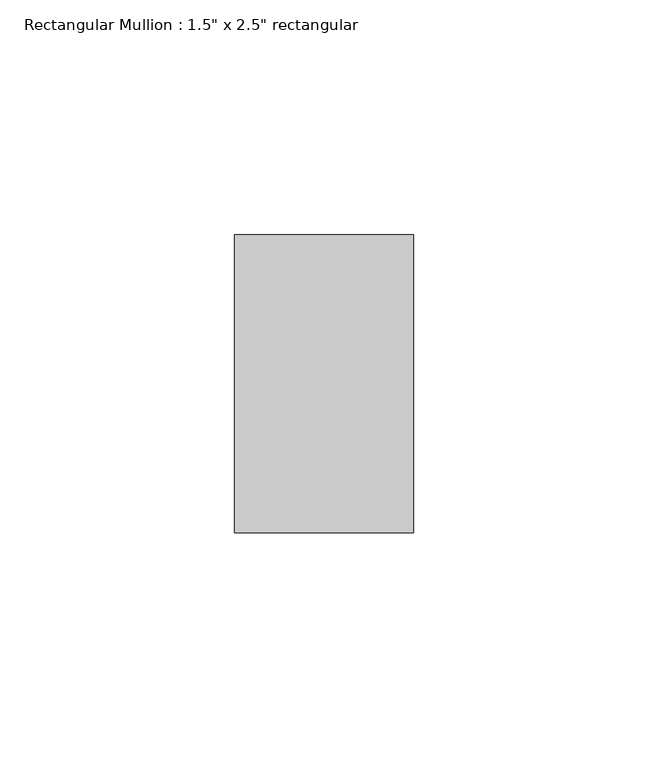
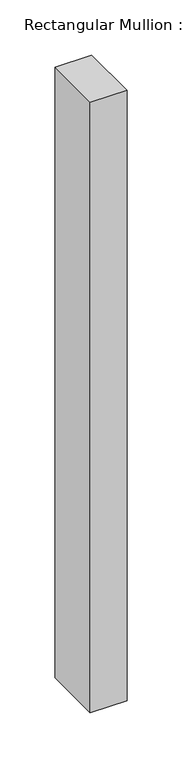
"""IFC4 building model written with IfcOpenShell, lengths in millimetres: member geometry."""

from ifc_helpers import new_model, si_unit, frame, origin, place, context, project, spatial, polyline, outline, extrude, source, transform, mapped, element, save


def member_7f78ed44(model_context):
    return source(origin(), model_context, "Body", "SweptSolid", [
        extrude(outline(polyline([(0.0, 31.75), (0.0, -31.75), (-38.1, -31.75), (-38.1, 31.75), (0.0, 31.75)])), frame((0.0, 0.0, -673.1), z_axis=(0.0, 0.0, 1.0), x_axis=(1.0, 0.0, 0.0)), (0.0, 0.0, 1.0), 673.1),
    ])


if __name__ == "__main__":
    model = new_model("IFC4")
    model_context = context("Model", 3, world=origin())
    ifc_project = project(units=[si_unit("LENGTHUNIT", "METRE", prefix="MILLI")], contexts=[model_context])
    site = spatial("IfcSite", under=ifc_project)
    building = spatial("IfcBuilding", under=site)
    placement = place(None, origin())
    member_shape = member_7f78ed44(model_context)
    element("IfcMember", 1, ObjectType="Rectangular Mullion : 1.5\" x 2.5\" rectangular", at=placement, inside=building, context=model_context, shape_type="MappedRepresentation", body=[
        mapped(member_shape, transform((0.0, 0.0, 0.0), x_axis=(1.0, 0.0, 0.0), y_axis=(0.0, 1.0, 0.0), z_axis=(0.0, 0.0, 1.0))),
    ])
    save(model, "model.ifc")

# Revit data of these elements
# Type "Rectangular Mullion : 1.5\" x 2.5\" rectangular"
#   built-in parameter 1007304 = 0.208333 (stored number, unit not read)
#   built-in parameter 1007301 = 0.0625 (stored number, unit not read)
#   built-in parameter 1007300 = 0.0625 (stored number, unit not read)
# Element 1 (IfcMember, "Rectangular Mullion : 1.5\" x 2.5\" rectangular")
#   Materials on its faces: "Leather - Black"
# Materials
#   "Leather - Black": class "Generic", colour RGB 40 40 40, transparency 0, Cost = 0
